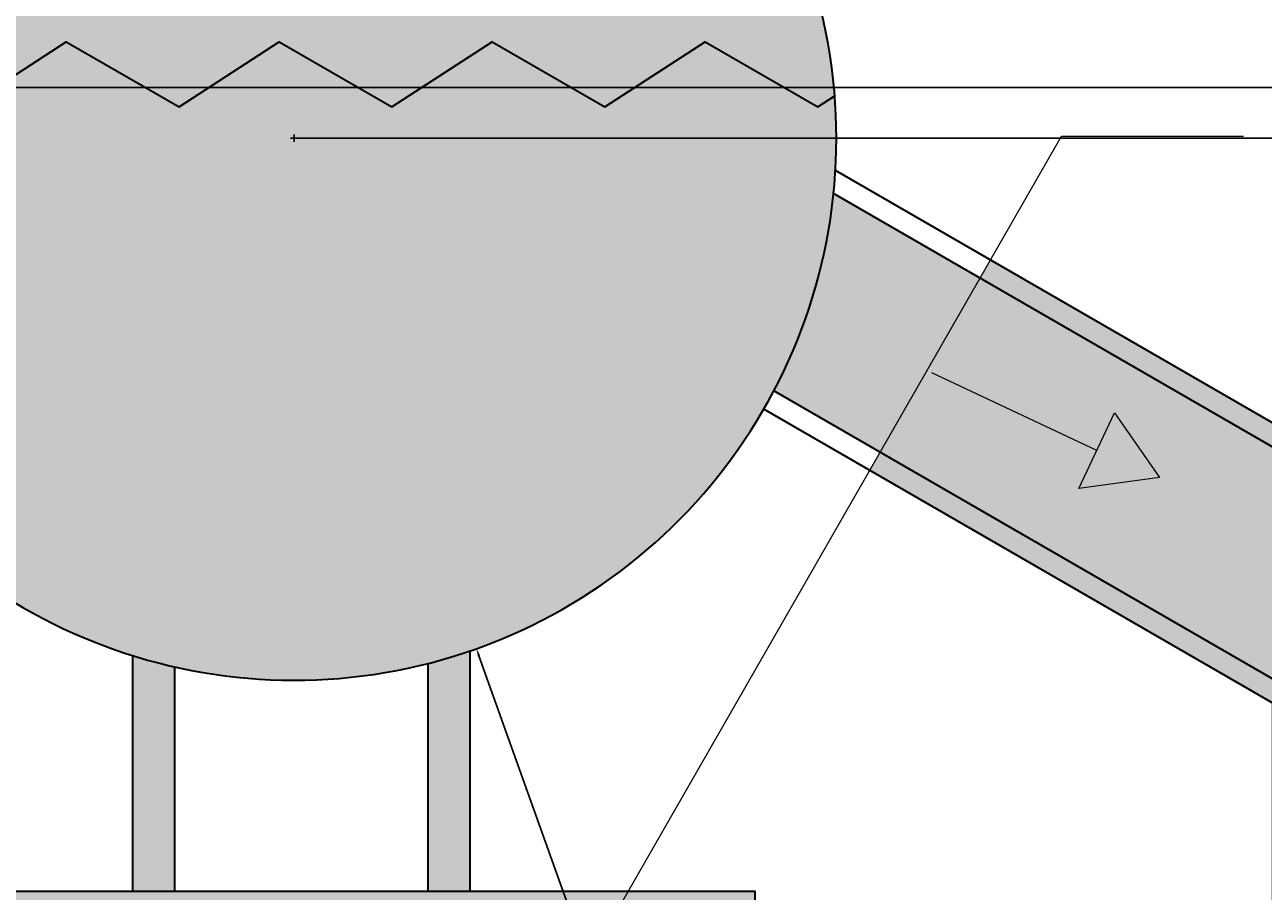
# Model space of a CAD drawing. Units: inches. Extents: x -1 to 292, y -3 to 199.
# Tile 47 of 52: x 237 to 267, y 81 to 101. Entities that reach past the tile are written whole.
import ezdxf

# ---------------------------------------------------------------- set-up
doc = ezdxf.new("R2010")
doc.units = ezdxf.units.IN
doc.header["$MEASUREMENT"] = 0
for name, color, linetype, lineweight in [('M-ANNO-LEAD', 2, 'Continuous', 18), ('M-ANNO-SYMB', 1, 'Continuous', 18), ('M-DIMS', 2, 'Continuous', 18), ('M-EQPM', 7, 'Continuous', 35), ('M-PATT', 8, 'Continuous', 13)]:
    doc.layers.add(name, color=color, linetype=linetype, lineweight=lineweight)
doc.styles.get("Standard").update_dxf_attribs({"font": 'arial.ttf'})
doc.dimstyles.get("Standard").update_dxf_attribs({"dimtxt": 0.18, "dimasz": 0.18, "dimexe": 0.18, "dimexo": 0.0625, "dimgap": 0.09, "dimtad": 0, "dimtih": 1, "dimtoh": 1, "dimdec": 4, "dimzin": 0, "dimdsep": 46, "dimtxsty": 'Standard', "dimcen": 0.09, "dimadec": 0, "dimazin": 0, "dimtfac": 1, "dimtdec": 4, "dimtofl": 0, "dimtmove": 0, "dimatfit": 3, "dimfxl": 1, "dimtolj": 1, "dimtzin": 0, "dimarcsym": 0})

# ---------------------------------------------------------------- blocks, each defined once
blk = doc.blocks.new('FLOW-ARROW-WATER')
blk.add_line((223.29, 53.741), (227.063, 51.564))
blk.add_lwpolyline([(222.79, 52.875), (221.849, 54.506), (223.79, 54.608)], close=True)
blk = doc.blocks.new('*D10')
at = {"layer": 'Defpoints', "color": 0, "transparency": 16777216}
for p in [(169.176, 99.774), (169.176, 43.391), (292.04, 43.391)]:
    blk.add_point(p, dxfattribs=at)
at = {"layer": 'M-DIMS', "color": 0, "lineweight": -2, "transparency": 16777216}
for p, q in [((169.239, 99.774), (292.22, 99.774)), ((292.04, 99.594), (292.04, 71.764)), ((292.04, 43.571), (292.04, 71.4)), ((169.239, 43.391), (292.22, 43.391))]:
    blk.add_line(p, q, dxfattribs=at)
at = {"layer": 'M-DIMS', "color": 0, "transparency": 16777216}
for points in [[(292.01, 99.594), (292.07, 99.594), (292.04, 99.774)], [(292.01, 43.571), (292.07, 43.571), (292.04, 43.391)]]:
    blk.add_solid(points, dxfattribs=at)
at = {"layer": 'M-DIMS', "color": 0, "transparency": 16777216, "insert": (292.04, 71.582), "char_height": 0.18, "attachment_point": 5}
blk.add_mtext('\\A1;56.38', dxfattribs=at)
blk = doc.blocks.new('*D25')
at = {"layer": 'Defpoints', "color": 0, "transparency": 16777216}
for p in [(215.241, 88.13), (273.066, 88.419), (273.066, -2.71)]:
    blk.add_point(p, dxfattribs=at)
at = {"layer": 'M-DIMS', "color": 0, "lineweight": -2, "transparency": 16777216}
for p, q in [((273.066, 88.357), (273.066, -2.89)), ((215.241, 88.068), (215.241, -2.89)), ((215.421, -2.71), (243.76, -2.71)), ((272.886, -2.71), (244.547, -2.71))]:
    blk.add_line(p, q, dxfattribs=at)
at = {"layer": 'M-DIMS', "color": 0, "transparency": 16777216}
for points in [[(215.421, -2.68), (215.421, -2.74), (215.241, -2.71)], [(272.886, -2.68), (272.886, -2.74), (273.066, -2.71)]]:
    blk.add_solid(points, dxfattribs=at)
at = {"layer": 'M-DIMS', "color": 0, "transparency": 16777216, "insert": (244.153, -2.71), "char_height": 0.18, "attachment_point": 5}
blk.add_mtext('\\A1;57.83', dxfattribs=at)
blk = doc.blocks.new('*D29')
at = {"layer": 'Defpoints', "color": 0, "transparency": 16777216}
for p in [(243.903, 98.567), (243.903, 44.598), (292.04, 44.598)]:
    blk.add_point(p, dxfattribs=at)
at = {"layer": 'M-DIMS', "color": 0, "lineweight": -2, "transparency": 16777216}
for p, q in [((243.966, 98.567), (292.22, 98.567)), ((292.04, 98.387), (292.04, 71.764)), ((292.04, 44.778), (292.04, 71.4)), ((243.966, 44.598), (292.22, 44.598))]:
    blk.add_line(p, q, dxfattribs=at)
at = {"layer": 'M-DIMS', "color": 0, "transparency": 16777216}
for points in [[(292.01, 98.387), (292.07, 98.387), (292.04, 98.567)], [(292.01, 44.778), (292.07, 44.778), (292.04, 44.598)]]:
    blk.add_solid(points, dxfattribs=at)
at = {"layer": 'M-DIMS', "color": 0, "transparency": 16777216, "insert": (292.04, 71.582), "char_height": 0.18, "attachment_point": 5}
blk.add_mtext('\\A1;53.97', dxfattribs=at)
blk = doc.blocks.new('*D33')
at = {"layer": 'Defpoints', "color": 0, "transparency": 16777216}
for p in [(242.955, 125.727), (292.04, 125.727), (237.933, 30.73)]:
    blk.add_point(p, dxfattribs=at)
at = {"layer": 'M-DIMS', "color": 0, "lineweight": -2, "transparency": 16777216}
for p, q in [((243.018, 125.727), (292.22, 125.727)), ((292.04, 125.547), (292.04, 78.41)), ((292.04, 30.91), (292.04, 78.046)), ((237.996, 30.73), (292.22, 30.73))]:
    blk.add_line(p, q, dxfattribs=at)
at = {"layer": 'M-DIMS', "color": 0, "transparency": 16777216}
for points in [[(292.01, 125.547), (292.07, 125.547), (292.04, 125.727)], [(292.01, 30.91), (292.07, 30.91), (292.04, 30.73)]]:
    blk.add_solid(points, dxfattribs=at)
at = {"layer": 'M-DIMS', "color": 0, "transparency": 16777216, "insert": (292.04, 78.228), "char_height": 0.18, "attachment_point": 5}
blk.add_mtext('\\A1;95', dxfattribs=at)
blk = doc.blocks.new('*D35')
at = {"layer": 'Defpoints', "color": 0, "transparency": 16777216}
for p in [(243.903, 98.567), (248.254, 86.374)]:
    blk.add_point(p, dxfattribs=at)
at = {"layer": 'M-DIMS', "color": 0, "lineweight": -2, "transparency": 16777216}
for p, q in [((243.813, 98.567), (243.993, 98.567)), ((243.903, 98.477), (243.903, 98.657)), ((250.864, 79.059), (248.314, 86.205)), ((251.044, 79.059), (250.864, 79.059))]:
    blk.add_line(p, q, dxfattribs=at)
at = {"layer": 'M-DIMS', "color": 0, "transparency": 16777216}
blk.add_solid([(248.343, 86.215), (248.286, 86.195), (248.254, 86.374)], dxfattribs=at)
at = {"layer": 'M-DIMS', "color": 0, "transparency": 16777216, "insert": (251.595, 79.059), "char_height": 0.18, "attachment_point": 5}
blk.add_mtext('\\A1;R12.945', dxfattribs=at)

msp = doc.modelspace()

# ---------------------------------------------------------------- hatches: boundary and pattern name
at = {"layer": 'M-PATT'}
h = msp.add_hatch(color=256, dxfattribs=at)
h.set_gradient(color1=(205, 32, 39), color2=(242, 113, 114), tint=1, name='CYLINDER')
h.paths.add_polyline_path([(243.5443, 100.87), (246.2365, 99.3157), (248.6299, 100.87), (251.3221, 99.3157), (253.7155, 100.87), (256.4077, 99.3157), (256.8092, 99.5764, 0.3682504), (244.9552, 111.4691), (244.9552, 109.7385), (248.4468, 109.7385), (248.4468, 107.2081), (239.4637, 107.2081), (239.4637, 109.7385), (242.9552, 109.7385), (242.9552, 111.4772, 0.1365835), (236.4209, 109.1305), (236.4209, 99.5466), (238.4587, 100.87), (241.1509, 99.3157)])
h.paths.add_polyline_path([(230.9797, 99.3157), (233.3731, 100.87), (234.9209, 99.9764), (234.9209, 107.8885, 0.1887049)])
h = msp.add_hatch(color=256, dxfattribs=at)
h.set_gradient(color1=(0, 255, 255), color2=(0, 255, 255), tint=1, name='CYLINDER')
h.paths.add_polyline_path([(256.8092, 99.5764), (256.4077, 99.3157), (253.7155, 100.87), (251.3221, 99.3157), (248.6299, 100.87), (246.2365, 99.3157), (243.5443, 100.87), (241.1509, 99.3157), (238.4587, 100.87), (236.4209, 99.5466), (236.4209, 97.1861), (234.9209, 97.1861), (234.9209, 99.9764), (233.3731, 100.87), (230.9797, 99.3157, 1.0704128)])
h.paths.add_polyline_path([(234.4549, 44.5975, 1), (253.3518, 44.5975, 1)])
h.paths.add_polyline_path([(235.4822, 48.8821), (220.034, 57.8011), (220.034, 85.363), (232.4507, 92.5318, -0.0853739), (231.0925, 96.7051), (215.7407, 87.8418), (215.7407, 55.3224), (234.4552, 44.5176, -0.0021162), (234.4549, 44.5975, -0.1182098)])
h.paths.add_polyline_path([(222.7904, 52.8755), (221.8492, 54.5058), (223.7904, 54.6075)], flags=16)
h.paths.add_polyline_path([(216.828, 66.8912), (217.7692, 68.5216), (218.828, 66.8912)], flags=16)
h.paths.add_polyline_path([(216.8084, 83.826), (217.7497, 85.4564), (218.8084, 83.826)], flags=16)
h.paths.add_polyline_path([(226.468, 92.8803), (228.3442, 93.0348), (227.6068, 91.2362)], flags=16)
h.paths.add_polyline_path([(272.5659, 88.1304), (260.2765, 95.2257), (259.0113, 93.0196), (263.0639, 91.1046), (263.4912, 92.0087), (264.5631, 90.4612), (262.6367, 90.2004), (263.0639, 91.1046), (259.0113, 93.0196), (257.8918, 91.0677), (267.7726, 85.363), (267.7726, 57.8011), (255.5043, 50.718), (257.0663, 46.085), (272.5659, 55.0337)])
h.paths.add_polyline_path([(263.6286, 51.5636), (261.7461, 51.5636), (262.6286, 53.2956)], flags=16)
h.paths.add_polyline_path([(269.8773, 65.3608), (268.8186, 66.9911), (270.8186, 66.9911)], flags=16)
h.paths.add_polyline_path([(269.8773, 80.8843), (268.8186, 82.5146), (270.8186, 82.5146)], flags=16)
h.paths.add_polyline_path([(255.5043, 50.718), (252.3244, 48.8821, -0.1182098), (253.3518, 44.5975, -0.0177685), (253.3279, 43.9266), (257.0663, 46.085)])
h.paths.add_polyline_path([(260.2765, 95.2257), (256.7809, 97.2439, -0.0959457), (255.356, 92.5318), (257.8918, 91.0677)])
h = msp.add_hatch(color=256, dxfattribs=at)
h.set_gradient(color1=(76, 38, 47), color2=(76, 38, 47), tint=1, name='CYLINDER')
h.paths.add_polyline_path([(267.2726, 58.0898), (255.3414, 51.2013), (255.5043, 50.718), (267.7726, 57.8011), (267.7726, 85.363), (257.8918, 91.0677), (257.643, 90.634), (267.2726, 85.0743)])
h.paths.add_polyline_path([(272.5659, 55.0337), (257.0663, 46.085), (257.2293, 45.6017), (273.0659, 54.745), (273.0659, 88.4191), (260.5253, 95.6595), (260.2765, 95.2257), (272.5659, 88.1304)])
h.paths.add_polyline_path([(215.2407, 55.0337), (234.4787, 43.9266, -0.0156517), (234.4552, 44.5176), (215.7407, 55.3224), (215.7407, 87.8418), (231.0925, 96.7051, -0.0104859), (231.0257, 97.2439), (215.2407, 88.1304)])
h.paths.add_polyline_path([(220.034, 57.8011), (235.4822, 48.8821, -0.0132367), (235.7207, 49.3218), (220.534, 58.0898), (220.534, 85.0743), (232.6923, 92.0939, -0.0096587), (232.4507, 92.5318), (220.034, 85.363)])
h = msp.add_hatch(color=256, dxfattribs=at)
h.set_gradient(color1=(0, 0, 255), color2=(0, 0, 255), tint=1, name='CYLINDER')
h.paths.add_polyline_path([(227.6068, 91.2362), (228.3442, 93.0348), (226.468, 92.8803)])
h.paths.add_polyline_path([(218.8084, 83.826), (217.7497, 85.4564), (216.8084, 83.826)])
h.paths.add_polyline_path([(262.6367, 90.2004), (264.5631, 90.4612), (263.4912, 92.0087)])
h.paths.add_polyline_path([(217.7692, 68.5216), (216.828, 66.8912), (218.828, 66.8912)])
h.paths.add_polyline_path([(223.7904, 54.6075), (221.8492, 54.5058), (222.7904, 52.8755)])
h.paths.add_polyline_path([(262.6286, 53.2956), (261.7461, 51.5636), (263.6286, 51.5636)])
h.paths.add_polyline_path([(268.8186, 82.5146), (269.8773, 80.8843), (270.8186, 82.5146)])
h.paths.add_polyline_path([(268.8186, 66.9911), (269.8773, 65.3608), (270.8186, 66.9911)])
h = msp.add_hatch(color=256, dxfattribs=at)
h.set_gradient(color1=(0, 255, 255), color2=(0, 255, 255), tint=1, name='CYLINDER')
h.paths.add_polyline_path([(241.0437, 75.7414), (240.0437, 75.7414), (240.0437, 67.4228), (241.0437, 67.4228)])
h.paths.add_polyline_path([(241.0437, 62.5821), (240.0437, 62.5821), (240.0437, 53.2217, -0.0283388), (241.0437, 53.6028)])
h.paths.add_polyline_path([(241.0437, 85.9411, -0.0200063), (240.0437, 86.21), (240.0437, 80.5821), (241.0437, 80.5821)])
h.paths.add_polyline_path([(248.0947, 86.3186, -0.0201581), (247.0947, 86.0208), (247.0947, 80.5821), (248.0947, 80.5821)])
h.paths.add_polyline_path([(244.5758, 75.7414), (243.5758, 75.7414), (243.5758, 67.4228), (244.5758, 67.4228)])
h.paths.add_polyline_path([(248.0947, 75.7414), (247.0947, 75.7414), (247.0947, 67.4228), (248.0947, 67.4228)])
h.paths.add_polyline_path([(248.0947, 62.5821), (247.0947, 62.5821), (247.0947, 53.4907, -0.0287763), (248.0947, 53.0654)])
h = msp.add_hatch(color=256, dxfattribs=at)
h.set_gradient(color1=(242, 103, 34), color2=(242, 103, 34), tint=1, name='CYLINDER')
h.paths.add_polyline_path([(232.9033, 62.5821), (254.9033, 62.5821), (254.9033, 80.5821), (251.8779, 80.5821), (250.2521, 77.7473), (252.0686, 77.7473), (252.0686, 65.4168), (235.7381, 65.4168), (235.7381, 77.7473), (250.2521, 77.7473), (251.8779, 80.5821), (232.9033, 80.5821)])

# ---------------------------------------------------------------- linework, layer by layer
at = {"layer": 'M-ANNO-LEAD'}
for p, q in [((247.5701, 73.0711), (262.2218, 98.6175)), ((262.2218, 98.6175), (266.5721, 98.6175))]:
    msp.add_line(p, q, dxfattribs=at)
at = {"layer": 'M-EQPM'}
for p, q in [((240.0437, 86.21), (240.0437, 80.5821)), ((248.0947, 86.3186), (248.0947, 80.5821)), ((241.0437, 85.9411), (241.0437, 80.5821)), ((247.0947, 86.0208), (247.0947, 80.5821))]:
    msp.add_line(p, q, dxfattribs=at)
for points in [[(236.4209, 99.5466), (238.4587, 100.87), (241.1509, 99.3157)], [(241.1509, 99.3157), (243.5443, 100.87), (246.2365, 99.3157)], [(246.2365, 99.3157), (248.6299, 100.87), (251.3221, 99.3157)], [(251.3221, 99.3157), (253.7155, 100.87), (256.4077, 99.3157)], [(256.4077, 99.3157), (256.8092, 99.5764)], [(253.2639, 43.3124), (273.0659, 54.745), (273.0659, 88.4191), (256.8257, 97.7954)], [(253.3279, 43.9266), (272.5659, 55.0337), (272.5659, 88.1304), (256.7809, 97.2439)], [(252.3359, 48.8887), (267.7726, 57.8011), (267.7726, 85.363), (255.356, 92.5318)], [(252.0859, 49.3218), (267.2726, 58.0898), (267.2726, 85.0743), (255.1143, 92.0939)]]:
    msp.add_lwpolyline(points, dxfattribs=at)
msp.add_lwpolyline([(232.9033, 80.5821), (254.9033, 80.5821), (254.9033, 62.5821), (232.9033, 62.5821)], close=True, dxfattribs=at)
msp.add_arc((243.9033, 98.5666), 12.9453, 133.93743, 85.33905, dxfattribs=at)

# ---------------------------------------------------------------- block references
at = {"layer": 'M-ANNO-SYMB', "rotation": 184.7076562269441}
msp.add_blockref('FLOW-ARROW-WATER', (481.1904, 162.9906), dxfattribs=at)

# ---------------------------------------------------------------- dimensions: what is measured, and where the dimension line sits
at = {"layer": 'M-DIMS'}
for base, p1, p2, override, picture, middle in [((292.0399, 125.7269), (237.9333, 30.7296), (242.9552, 125.7269), {"dimdec": 0, "dimlfac": 1, "dimrnd": 0, "dimzin": 0, "dimdsep": 46, "dimlunit": 2}, '*D33', (292.0399, 78.2282)), ((292.0399, 43.3906), (169.176, 99.7735), (169.176, 43.3906), {"dimdec": 2, "dimlfac": 1, "dimrnd": 0, "dimzin": 0, "dimdsep": 46, "dimlunit": 2}, '*D10', (292.0399, 71.5821)), ((292.0399, 44.5975), (243.9033, 98.5666), (243.9033, 44.5975), {"dimdec": 2, "dimlfac": 1, "dimrnd": 0, "dimzin": 0, "dimdsep": 46, "dimlunit": 2}, '*D29', (292.0399, 71.5821))]:
    dim = msp.add_linear_dim(base=base, p1=p1, p2=p2, angle=90, dimstyle='Standard', override=override, dxfattribs=at)
    dim.commit()
    dim.dimension.update_dxf_attribs({"geometry": picture, "text_midpoint": middle})
dim = msp.add_radius_dim(center=(243.9033, 98.5666), mpoint=(248.2539, 86.3742), dimstyle='Standard', override={"dimdec": 3, "dimlfac": 1, "dimrnd": 0, "dimzin": 0, "dimdsep": 46, "dimlunit": 2}, dxfattribs=at)
dim.commit()
dim.dimension.update_dxf_attribs({"geometry": '*D35', "text_midpoint": (251.5947, 79.0588), "dimtype": 164})
dim = msp.add_linear_dim(base=(273.0659, -2.7104), p1=(215.2407, 88.1304), p2=(273.0659, 88.4191), dimstyle='Standard', override={"dimdec": 2, "dimlfac": 1, "dimrnd": 0, "dimzin": 0, "dimdsep": 46, "dimlunit": 2}, dxfattribs=at)
dim.commit()
dim.dimension.update_dxf_attribs({"geometry": '*D25', "text_midpoint": (244.1533, -2.7104)})

doc.saveas('drawing.dxf')
